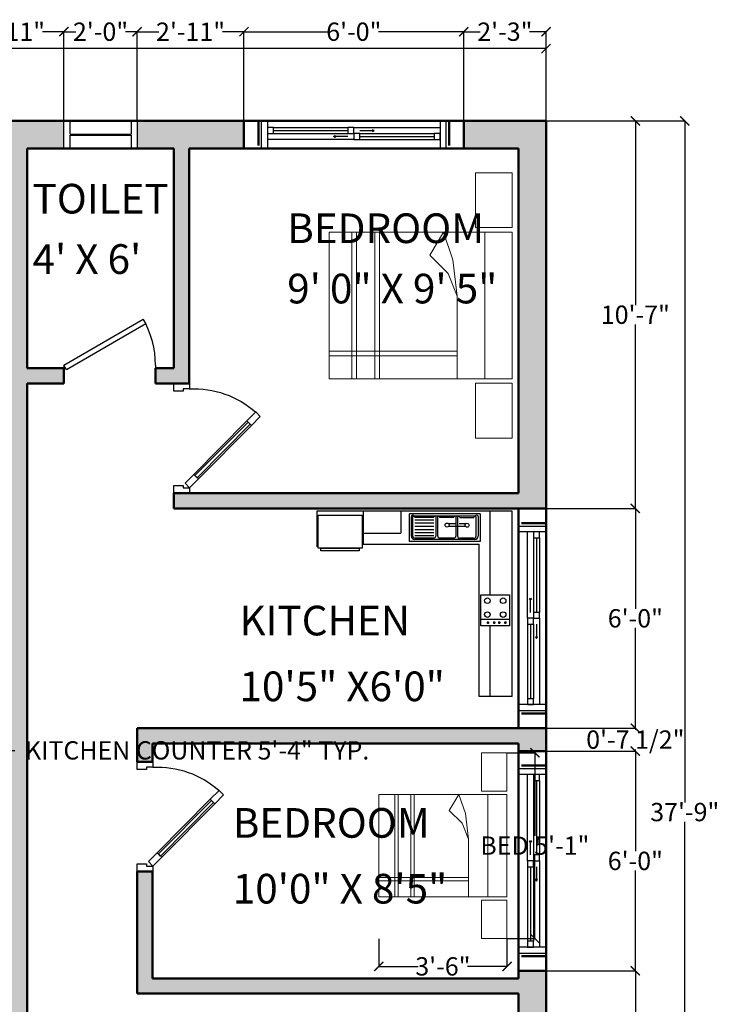
# Model space of a CAD drawing. Units: inches. Extents: x 2278 to 7495, y -71 to 1198.
# Tile 7 of 44: x 3076 to 3306, y 873 to 1195. Entities that reach past the tile are written whole.
import ezdxf

# ---------------------------------------------------------------- set-up
doc = ezdxf.new("R2010")
doc.units = ezdxf.units.IN
doc.header["$MEASUREMENT"] = 0
for name, color, linetype, lineweight in [('A-ANNO-DIMS', 2, 'Continuous', 18), ('A-AREA-IDEN', 3, 'Continuous', 18), ('A-Door', 3, 'Continuous', 25), ('A-FLOR-FIXT', 9, 'Continuous', 18), ('A-FURN', 8, 'Continuous', 18), ('A-Glaz', 4, 'Continuous', 25), ('A-Wall', 7, 'Continuous', 50), ('A-WALL-PATT', 8, 'Continuous', 18)]:
    doc.layers.add(name, color=color, linetype=linetype, lineweight=lineweight)
doc.layers.add('TEFRIŞ', color=11, linetype='Continuous')
doc.styles.get("Standard").update_dxf_attribs({"font": 'arial.ttf'})
doc.dimstyles.get("Standard").update_dxf_attribs({"dimtxt": 6, "dimasz": 3, "dimexe": 0.18, "dimexo": 0.0625, "dimgap": 0.09, "dimtad": 0, "dimtih": 1, "dimtoh": 1, "dimdec": 0, "dimzin": 0, "dimdsep": 46, "dimlunit": 3, "dimtxsty": 'Standard', "dimblk": 'ARCHTICK', "dimcen": 0.09, "dimadec": 0, "dimazin": 0, "dimtfac": 1, "dimtdec": 0, "dimtofl": 0, "dimtmove": 0, "dimatfit": 3, "dimfxl": 1, "dimtolj": 1, "dimtzin": 0, "dimarcsym": 0})

# ---------------------------------------------------------------- blocks, each defined once
blk = doc.blocks.new('A$C1DF4181C')
blk.add_lwpolyline([(120, 128), (460.7, 466.1), (432.5, 494.5), (91.8, 156.4)], close=True)
blk.add_arc((72.4, 128.7), 593.3, 357.23132, 41.49368)
at = {"layer": 'A-Door'}
for points in [[(517.5, 522.4), (460.7, 466.1), (432.5, 494.5), (489.3, 550.8)], [(63.2, 71.6), (120, 128), (91.8, 156.4), (35, 100)], [(35, 100), (0, 100), (0, 0), (50, 0), (50, 50), (50, 60), (35, 60)], [(665, 100), (665, 60), (650, 60), (650, 50), (650, 0), (700, 0), (700, 100)]]:
    blk.add_lwpolyline(points, close=True, dxfattribs=at)
at = {"layer": 'A-Glaz'}
blk.add_lwpolyline([(112.9, 135.1), (453.6, 473.2), (439.5, 487.4), (98.8, 149.3)], close=True, dxfattribs=at)
at = {"layer": 'A-Wall'}
for p, q in [((0, 0), (0, 100)), ((0, 100), (0, 0)), ((700, 0), (700, 100)), ((700, 0), (700, 100))]:
    blk.add_line(p, q, dxfattribs=at)
blk = doc.blocks.new('*U4')
for p, q in [((0, 0), (0, -6)), ((30, 0), (30, -6))]:
    blk.add_line(p, q)
blk.add_lwpolyline([(0, 0), (25.98, 15), (26.86, 13.48), (0.87, -1.52)], close=True)
blk.add_arc((0, 0), 30, 0, 30)
blk = doc.blocks.new('BED-160')
at = {"color": 0}
for p, q in [((-0.45, 2.35), (-0.45, 2.95)), ((-0.45, 2.95), (-0.05, 2.95)), ((-0.05, 2.95), (-0.05, 2.35)), ((-2.05, 2.3), (-0.05, 2.3)), ((-2.05, 0.7), (-2.05, 2.3)), ((-1.8, 0.7), (-1.8, 2.3)), ((-1.75, 0.7), (-1.75, 2.3)), ((-1.55, 0.7), (-1.55, 2.3)), ((-1.5, 0.7), (-1.5, 2.3)), ((-0.8, 2.3), (-0.95, 2.05)), ((-0.8, 2.3), (-0.7, 2)), ((-0.05, 2.35), (-0.45, 2.35)), ((-0.35, 0.7), (-0.35, 2.3)), ((-0.05, 2.3), (-0.05, 0.7)), ((-0.95, 2.05), (-0.75, 1.85)), ((-0.7, 2), (-0.65, 1.6)), ((-0.75, 1.85), (-0.65, 1.6)), ((-0.65, 1.6), (-0.65, 0.7)), ((-0.65, 1), (-2.05, 1)), ((-0.65, 0.95), (-2.05, 0.95)), ((-0.05, 0.7), (-2.05, 0.7)), ((-0.45, 0.65), (-0.05, 0.65)), ((-0.45, 0.05), (-0.45, 0.65)), ((-0.05, 0.65), (-0.05, 0.05)), ((-0.05, 0.05), (-0.45, 0.05))]:
    blk.add_line(p, q, dxfattribs=at)
blk = doc.blocks.new('A$C008029BD')
at = {"layer": 'TEFRIŞ', "ltscale": 0.05}
for p, q in [((0, 0), (0, -3.55)), ((3.37, 0), (0, 0)), ((3.37, 0), (3.37, -0.6)), ((1.522, -0.4), (0, -0.4)), ((3.37, -0.4), (2.083, -0.4)), ((0.05, -0.581), (0.05, -1.869)), ((0.05, -0.581), (0.55, -0.581)), ((0.086, -1.773), (0.086, -0.677)), ((0.096, -0.617), (0.454, -0.617)), ((0.099, -0.659), (0.457, -0.659)), ((0.113, -0.954), (0.113, -0.695)), ((0.493, -0.695), (0.493, -0.954)), ((0.514, -0.677), (0.514, -1.773)), ((0.55, -0.581), (0.55, -1.869)), ((0.6, -2.71), (0.6, -0.6)), ((3.37, -0.6), (0.6, -0.6)), ((0.23, -0.846), (0.229, -0.967)), ((0.28, -0.846), (0.277, -1.158)), ((0.096, -1.024), (0.454, -1.024)), ((0.457, -0.99), (0.099, -0.99)), ((0.11, -1.319), (0.11, -1.06)), ((0.228, -1.02), (0.227, -1.159)), ((0.49, -1.06), (0.49, -1.319)), ((0.454, -1.355), (0.096, -1.355)), ((0.096, -1.391), (0.454, -1.391)), ((0.11, -1.773), (0.11, -1.427)), ((0.154, -1.773), (0.154, -1.427)), ((0.214, -1.773), (0.214, -1.427)), ((0.274, -1.773), (0.274, -1.427)), ((0.334, -1.773), (0.334, -1.427)), ((0.39, -1.773), (0.39, -1.427)), ((0.444, -1.773), (0.444, -1.427)), ((0.49, -1.427), (0.49, -1.773)), ((0.55, -1.869), (0.05, -1.869)), ((0.454, -1.809), (0.096, -1.809)), ((0.454, -1.833), (0.096, -1.833)), ((0, -2.025), (0.4, -2.025)), ((0.4, -2.71), (0.4, -2.025)), ((0, -2.71), (0.6, -2.71)), ((0, -3.55), (0.65, -3.55))]:
    blk.add_line(p, q, dxfattribs=at)
at = {"layer": 'TEFRIŞ'}
blk.add_line((1.969, -0.05), (1.969, -0.572), dxfattribs=at)
at = {"layer": 'TEFRIŞ', "ltscale": 0.05}
for points in [[(1.522, -0.05), (2.083, -0.05), (2.083, -0.572), (1.522, -0.572)], [(0.67, -2.73), (0.67, -3.53), (0.07, -3.53), (0.07, -2.73)], [(0.72, -2.78), (0.72, -3.48), (0.67, -3.48), (0.67, -2.78)]]:
    blk.add_lwpolyline(points, close=True, dxfattribs=at)
at = {"layer": 'TEFRIŞ', "const_width": 0.025}
for points in [[(2.014, -0.123, 1), (2.039, -0.123, 1)], [(2.014, -0.236, 1), (2.039, -0.236, 1)], [(2.014, -0.327, 1), (2.039, -0.327, 1)], [(2.014, -0.44, 1), (2.039, -0.44, 1)]]:
    blk.add_lwpolyline(points, format="xyb", close=True, dxfattribs=at)
at = {"layer": 'TEFRIŞ', "ltscale": 0.05}
for centre, radius in [((1.628, -0.164), 0.0505), ((1.628, -0.45), 0.0505), ((0.255, -0.82), 0.036), ((0.252, -1.184), 0.036)]:
    blk.add_circle(centre, radius, dxfattribs=at)
at = {"layer": 'TEFRIŞ'}
for centre in [(1.88, -0.164), (1.88, -0.45)]:
    blk.add_circle(centre, 0.0505, dxfattribs=at)
at = {"layer": 'TEFRIŞ', "ltscale": 0.05}
for centre, radius, start, end in [((0.108, -0.649), 0.0351, 110.4976, 230.5777), ((0.118, -0.673), 0.023, 143.9853, 258.5157), ((0.454, -0.677), 0.06, 0, 90), ((0.457, -0.695), 0.036, 0, 90), ((0.115, -1.038), 0.023, 143.9853, 258.5157), ((0.118, -0.976), 0.023, 101.4843, 216.0147), ((0.454, -1.06), 0.036, 0, 90), ((0.457, -0.954), 0.036, 270, 0), ((0.115, -1.341), 0.023, 101.4843, 216.0147), ((0.115, -1.405), 0.023, 143.9853, 258.5157), ((0.454, -1.319), 0.036, 270, 0), ((0.454, -1.427), 0.036, 0, 90), ((0.108, -1.801), 0.0351, 129.4223, 249.5024), ((0.115, -1.796), 0.023, 101.4843, 216.0147), ((0.454, -1.773), 0.06, 270, 0), ((0.454, -1.773), 0.036, 270, 0)]:
    blk.add_arc(centre, radius, start, end, dxfattribs=at)
blk = doc.blocks.new('_ArchTick')
at = {"color": 0, "linetype": 'ByBlock', "const_width": 0.15}
blk.add_lwpolyline([(-0.5, -0.5), (0.5, 0.5)], dxfattribs=at)
blk = doc.blocks.new('*D35')
at = {"layer": 'A-ANNO-DIMS', "color": 0, "lineweight": -2, "transparency": 16777216}
for p, q in [((3248.99, 1162.26), (3294.56, 1162.26)), ((3294.38, 1162.26), (3294.38, 938.91)), ((3294.38, 709.26), (3294.38, 932.6)), ((3248.99, 709.26), (3294.56, 709.26))]:
    blk.add_line(p, q, dxfattribs=at)
at = {"layer": 'Defpoints', "color": 0, "transparency": 16777216}
for p in [(3248.93, 1162.26), (3248.93, 709.26), (3294.38, 709.26)]:
    blk.add_point(p, dxfattribs=at)
at = {"layer": 'A-ANNO-DIMS', "color": 0, "lineweight": -2, "transparency": 16777216, "xscale": 3, "yscale": 3, "zscale": 3}
for p, rotation in [((3294.38, 1162.26), 90), ((3294.38, 709.26), 270)]:
    blk.add_blockref('_ArchTick', p, dxfattribs=dict(at, rotation=rotation))
at = {"layer": 'A-ANNO-DIMS', "color": 0, "transparency": 16777216, "insert": (3294.38, 935.76), "char_height": 6, "attachment_point": 5}
blk.add_mtext('\\A1;37\'-9"', dxfattribs=at)
blk = doc.blocks.new('*D36')
at = {"layer": 'A-ANNO-DIMS', "color": 0, "lineweight": -2, "transparency": 16777216}
for p, q in [((2845.93, 1162.32), (2845.93, 1186.15)), ((2845.93, 1185.97), (3037.04, 1185.97)), ((3248.93, 1185.97), (3057.82, 1185.97)), ((3248.93, 1162.32), (3248.93, 1186.15))]:
    blk.add_line(p, q, dxfattribs=at)
at = {"layer": 'Defpoints', "color": 0, "transparency": 16777216}
for p in [(3248.93, 1185.97), (2845.93, 1162.26), (3248.93, 1162.26)]:
    blk.add_point(p, dxfattribs=at)
at = {"layer": 'A-ANNO-DIMS', "color": 0, "lineweight": -2, "transparency": 16777216, "xscale": 3, "yscale": 3, "zscale": 3, "rotation": 180}
blk.add_blockref('_ArchTick', (2845.93, 1185.97), dxfattribs=at)
at = {"layer": 'A-ANNO-DIMS', "color": 0, "lineweight": -2, "transparency": 16777216, "xscale": 3, "yscale": 3, "zscale": 3}
blk.add_blockref('_ArchTick', (3248.93, 1185.97), dxfattribs=at)
at = {"layer": 'A-ANNO-DIMS', "color": 0, "transparency": 16777216, "insert": (3047.43, 1185.97), "char_height": 6, "attachment_point": 5}
blk.add_mtext('\\A1;33\'-7"', dxfattribs=at)
blk = doc.blocks.new('*D51')
at = {"layer": 'A-ANNO-DIMS', "color": 0, "lineweight": -2, "transparency": 16777216}
for p, q in [((3236.18, 955.22), (3245.43, 955.22)), ((3245.25, 955.22), (3245.25, 927.93)), ((3245.25, 894.32), (3245.25, 921.62)), ((3236.18, 894.32), (3245.43, 894.32))]:
    blk.add_line(p, q, dxfattribs=at)
at = {"layer": 'Defpoints', "color": 0, "transparency": 16777216}
for p in [(3236.12, 955.22), (3245.25, 955.22), (3236.12, 894.32)]:
    blk.add_point(p, dxfattribs=at)
at = {"layer": 'A-ANNO-DIMS', "color": 0, "lineweight": -2, "transparency": 16777216, "xscale": 3, "yscale": 3, "zscale": 3}
for p, rotation in [((3245.25, 955.22), 90), ((3245.25, 894.32), 270)]:
    blk.add_blockref('_ArchTick', p, dxfattribs=dict(at, rotation=rotation))
at = {"layer": 'A-ANNO-DIMS', "color": 0, "transparency": 16777216, "insert": (3245.25, 924.77), "char_height": 6, "attachment_point": 5}
blk.add_mtext('\\A1;BED 5\'-1"', dxfattribs=at)
blk = doc.blocks.new('*D52')
at = {"layer": 'A-ANNO-DIMS', "color": 0, "lineweight": -2, "transparency": 16777216}
for p, q in [((3194.12, 894.26), (3194.12, 885.01)), ((3236.12, 894.26), (3236.12, 885.01)), ((3194.12, 885.19), (3207.06, 885.19)), ((3236.12, 885.19), (3223.18, 885.19))]:
    blk.add_line(p, q, dxfattribs=at)
at = {"layer": 'Defpoints', "color": 0, "transparency": 16777216}
for p in [(3194.12, 894.32), (3236.12, 894.32), (3236.12, 885.19)]:
    blk.add_point(p, dxfattribs=at)
at = {"layer": 'A-ANNO-DIMS', "color": 0, "lineweight": -2, "transparency": 16777216, "xscale": 3, "yscale": 3, "zscale": 3, "rotation": 180}
blk.add_blockref('_ArchTick', (3194.12, 885.19), dxfattribs=at)
at = {"layer": 'A-ANNO-DIMS', "color": 0, "lineweight": -2, "transparency": 16777216, "xscale": 3, "yscale": 3, "zscale": 3}
blk.add_blockref('_ArchTick', (3236.12, 885.19), dxfattribs=at)
at = {"layer": 'A-ANNO-DIMS', "color": 0, "transparency": 16777216, "insert": (3215.12, 885.19), "char_height": 6, "attachment_point": 5}
blk.add_mtext('\\A1;3\'-6"', dxfattribs=at)
blk = doc.blocks.new('*D53')
at = {"layer": 'A-ANNO-DIMS', "color": 0, "lineweight": -2, "transparency": 16777216}
for p, q in [((3007.93, 965.51), (3007.93, 955.8)), ((3071.89, 965.51), (3071.89, 955.8)), ((3007.93, 955.98), (3071.89, 955.98)), ((3071.89, 955.98), (3074.89, 955.98))]:
    blk.add_line(p, q, dxfattribs=at)
at = {"layer": 'Defpoints', "color": 0, "transparency": 16777216}
for p in [(3007.93, 965.57), (3071.89, 965.57), (3071.89, 955.98)]:
    blk.add_point(p, dxfattribs=at)
at = {"layer": 'A-ANNO-DIMS', "color": 0, "lineweight": -2, "transparency": 16777216, "xscale": 3, "yscale": 3, "zscale": 3, "rotation": 180}
blk.add_blockref('_ArchTick', (3007.93, 955.98), dxfattribs=at)
at = {"layer": 'A-ANNO-DIMS', "color": 0, "lineweight": -2, "transparency": 16777216, "xscale": 3, "yscale": 3, "zscale": 3}
blk.add_blockref('_ArchTick', (3071.89, 955.98), dxfattribs=at)
at = {"layer": 'A-ANNO-DIMS', "color": 0, "transparency": 16777216, "insert": (3134.58, 955.98), "char_height": 6, "attachment_point": 5}
blk.add_mtext('\\A1;KITCHEN COUNTER 5\'-4" TYP.', dxfattribs=at)
blk = doc.blocks.new('*D81')
at = {"layer": 'A-ANNO-DIMS', "color": 0, "lineweight": -2, "transparency": 16777216}
for p, q in [((3055.93, 1162.32), (3055.93, 1191.69)), ((3055.93, 1191.51), (3062.98, 1191.51)), ((3090.93, 1191.51), (3083.88, 1191.51)), ((3090.93, 1162.32), (3090.93, 1191.69))]:
    blk.add_line(p, q, dxfattribs=at)
at = {"layer": 'Defpoints', "color": 0, "transparency": 16777216}
for p in [(3090.93, 1191.51), (3055.93, 1162.26), (3090.93, 1162.26)]:
    blk.add_point(p, dxfattribs=at)
at = {"layer": 'A-ANNO-DIMS', "color": 0, "lineweight": -2, "transparency": 16777216, "xscale": 3, "yscale": 3, "zscale": 3, "rotation": 180}
blk.add_blockref('_ArchTick', (3055.93, 1191.51), dxfattribs=at)
at = {"layer": 'A-ANNO-DIMS', "color": 0, "lineweight": -2, "transparency": 16777216, "xscale": 3, "yscale": 3, "zscale": 3}
blk.add_blockref('_ArchTick', (3090.93, 1191.51), dxfattribs=at)
at = {"layer": 'A-ANNO-DIMS', "color": 0, "transparency": 16777216, "insert": (3073.43, 1191.51), "char_height": 6, "attachment_point": 5}
blk.add_mtext('\\A1;2\'-11"', dxfattribs=at)
blk = doc.blocks.new('*D82')
at = {"layer": 'A-ANNO-DIMS', "color": 0, "lineweight": -2, "transparency": 16777216}
for p, q in [((3090.93, 1162.32), (3090.93, 1191.69)), ((3090.93, 1191.51), (3094.81, 1191.51)), ((3114.93, 1191.51), (3111.05, 1191.51)), ((3114.93, 1162.32), (3114.93, 1191.69))]:
    blk.add_line(p, q, dxfattribs=at)
at = {"layer": 'Defpoints', "color": 0, "transparency": 16777216}
for p in [(3114.93, 1191.51), (3090.93, 1162.26), (3114.93, 1162.26)]:
    blk.add_point(p, dxfattribs=at)
at = {"layer": 'A-ANNO-DIMS', "color": 0, "lineweight": -2, "transparency": 16777216, "xscale": 3, "yscale": 3, "zscale": 3, "rotation": 180}
blk.add_blockref('_ArchTick', (3090.93, 1191.51), dxfattribs=at)
at = {"layer": 'A-ANNO-DIMS', "color": 0, "lineweight": -2, "transparency": 16777216, "xscale": 3, "yscale": 3, "zscale": 3}
blk.add_blockref('_ArchTick', (3114.93, 1191.51), dxfattribs=at)
at = {"layer": 'A-ANNO-DIMS', "color": 0, "transparency": 16777216, "insert": (3102.93, 1191.51), "char_height": 6, "attachment_point": 5}
blk.add_mtext('\\A1;2\'-0"', dxfattribs=at)
blk = doc.blocks.new('*D83')
at = {"layer": 'A-ANNO-DIMS', "color": 0, "lineweight": -2, "transparency": 16777216}
for p, q in [((3114.93, 1162.32), (3114.93, 1191.69)), ((3114.93, 1191.51), (3121.98, 1191.51)), ((3149.93, 1191.51), (3142.88, 1191.51)), ((3149.93, 1162.32), (3149.93, 1191.69))]:
    blk.add_line(p, q, dxfattribs=at)
at = {"layer": 'Defpoints', "color": 0, "transparency": 16777216}
for p in [(3149.93, 1191.51), (3114.93, 1162.26), (3149.93, 1162.26)]:
    blk.add_point(p, dxfattribs=at)
at = {"layer": 'A-ANNO-DIMS', "color": 0, "lineweight": -2, "transparency": 16777216, "xscale": 3, "yscale": 3, "zscale": 3, "rotation": 180}
blk.add_blockref('_ArchTick', (3114.93, 1191.51), dxfattribs=at)
at = {"layer": 'A-ANNO-DIMS', "color": 0, "lineweight": -2, "transparency": 16777216, "xscale": 3, "yscale": 3, "zscale": 3}
blk.add_blockref('_ArchTick', (3149.93, 1191.51), dxfattribs=at)
at = {"layer": 'A-ANNO-DIMS', "color": 0, "transparency": 16777216, "insert": (3132.43, 1191.51), "char_height": 6, "attachment_point": 5}
blk.add_mtext('\\A1;2\'-11"', dxfattribs=at)
blk = doc.blocks.new('*D84')
at = {"layer": 'A-ANNO-DIMS', "color": 0, "lineweight": -2, "transparency": 16777216}
for p, q in [((3149.93, 1162.32), (3149.93, 1191.69)), ((3149.93, 1191.51), (3177.85, 1191.51)), ((3221.93, 1191.51), (3194.01, 1191.51)), ((3221.93, 1162.32), (3221.93, 1191.69))]:
    blk.add_line(p, q, dxfattribs=at)
at = {"layer": 'Defpoints', "color": 0, "transparency": 16777216}
for p in [(3221.93, 1191.51), (3149.93, 1162.26), (3221.93, 1162.26)]:
    blk.add_point(p, dxfattribs=at)
at = {"layer": 'A-ANNO-DIMS', "color": 0, "lineweight": -2, "transparency": 16777216, "xscale": 3, "yscale": 3, "zscale": 3, "rotation": 180}
blk.add_blockref('_ArchTick', (3149.93, 1191.51), dxfattribs=at)
at = {"layer": 'A-ANNO-DIMS', "color": 0, "lineweight": -2, "transparency": 16777216, "xscale": 3, "yscale": 3, "zscale": 3}
blk.add_blockref('_ArchTick', (3221.93, 1191.51), dxfattribs=at)
at = {"layer": 'A-ANNO-DIMS', "color": 0, "transparency": 16777216, "insert": (3185.93, 1191.51), "char_height": 6, "attachment_point": 5}
blk.add_mtext('\\A1;6\'-0"', dxfattribs=at)
blk = doc.blocks.new('*D85')
at = {"layer": 'A-ANNO-DIMS', "color": 0, "lineweight": -2, "transparency": 16777216}
for p, q in [((3221.93, 1162.32), (3221.93, 1191.69)), ((3221.93, 1191.51), (3227.31, 1191.51)), ((3248.93, 1191.51), (3243.55, 1191.51)), ((3248.93, 1162.32), (3248.93, 1191.69))]:
    blk.add_line(p, q, dxfattribs=at)
at = {"layer": 'Defpoints', "color": 0, "transparency": 16777216}
for p in [(3248.93, 1191.51), (3221.93, 1162.26), (3248.93, 1162.26)]:
    blk.add_point(p, dxfattribs=at)
at = {"layer": 'A-ANNO-DIMS', "color": 0, "lineweight": -2, "transparency": 16777216, "xscale": 3, "yscale": 3, "zscale": 3, "rotation": 180}
blk.add_blockref('_ArchTick', (3221.93, 1191.51), dxfattribs=at)
at = {"layer": 'A-ANNO-DIMS', "color": 0, "lineweight": -2, "transparency": 16777216, "xscale": 3, "yscale": 3, "zscale": 3}
blk.add_blockref('_ArchTick', (3248.93, 1191.51), dxfattribs=at)
at = {"layer": 'A-ANNO-DIMS', "color": 0, "transparency": 16777216, "insert": (3235.43, 1191.51), "char_height": 6, "attachment_point": 5}
blk.add_mtext('\\A1;2\'-3"', dxfattribs=at)
blk = doc.blocks.new('*D86')
at = {"layer": 'A-ANNO-DIMS', "color": 0, "lineweight": -2, "transparency": 16777216}
for p, q in [((3248.99, 1162.26), (3278.36, 1162.26)), ((3278.18, 1162.26), (3278.18, 1101.91)), ((3278.18, 1035.26), (3278.18, 1095.6)), ((3248.99, 1035.26), (3278.36, 1035.26))]:
    blk.add_line(p, q, dxfattribs=at)
at = {"layer": 'Defpoints', "color": 0, "transparency": 16777216}
for p in [(3248.93, 1162.26), (3248.93, 1035.26), (3278.18, 1035.26)]:
    blk.add_point(p, dxfattribs=at)
at = {"layer": 'A-ANNO-DIMS', "color": 0, "lineweight": -2, "transparency": 16777216, "xscale": 3, "yscale": 3, "zscale": 3}
for p, rotation in [((3278.18, 1162.26), 90), ((3278.18, 1035.26), 270)]:
    blk.add_blockref('_ArchTick', p, dxfattribs=dict(at, rotation=rotation))
at = {"layer": 'A-ANNO-DIMS', "color": 0, "transparency": 16777216, "insert": (3278.18, 1098.76), "char_height": 6, "attachment_point": 5}
blk.add_mtext('\\A1;10\'-7"', dxfattribs=at)
blk = doc.blocks.new('*D87')
at = {"layer": 'A-ANNO-DIMS', "color": 0, "lineweight": -2, "transparency": 16777216}
for p, q in [((3248.99, 1035.26), (3278.36, 1035.26)), ((3278.18, 1035.26), (3278.18, 1002.41)), ((3278.18, 963.26), (3278.18, 996.1)), ((3248.99, 963.26), (3278.36, 963.26))]:
    blk.add_line(p, q, dxfattribs=at)
at = {"layer": 'Defpoints', "color": 0, "transparency": 16777216}
for p in [(3248.93, 1035.26), (3248.93, 963.26), (3278.18, 963.26)]:
    blk.add_point(p, dxfattribs=at)
at = {"layer": 'A-ANNO-DIMS', "color": 0, "lineweight": -2, "transparency": 16777216, "xscale": 3, "yscale": 3, "zscale": 3}
for p, rotation in [((3278.18, 1035.26), 90), ((3278.18, 963.26), 270)]:
    blk.add_blockref('_ArchTick', p, dxfattribs=dict(at, rotation=rotation))
at = {"layer": 'A-ANNO-DIMS', "color": 0, "transparency": 16777216, "insert": (3278.18, 999.26), "char_height": 6, "attachment_point": 5}
blk.add_mtext('\\A1;6\'-0"', dxfattribs=at)
blk = doc.blocks.new('*D88')
at = {"layer": 'A-ANNO-DIMS', "color": 0, "lineweight": -2, "transparency": 16777216}
for p, q in [((3248.99, 963.26), (3278.36, 963.26)), ((3278.18, 963.26), (3278.18, 962.7)), ((3248.99, 955.76), (3278.36, 955.76)), ((3278.18, 955.76), (3278.18, 956.31))]:
    blk.add_line(p, q, dxfattribs=at)
at = {"layer": 'Defpoints', "color": 0, "transparency": 16777216}
for p in [(3248.93, 963.26), (3248.93, 955.76), (3278.18, 955.76)]:
    blk.add_point(p, dxfattribs=at)
at = {"layer": 'A-ANNO-DIMS', "color": 0, "lineweight": -2, "transparency": 16777216, "xscale": 3, "yscale": 3, "zscale": 3}
for p, rotation in [((3278.18, 963.26), 90), ((3278.18, 955.76), 270)]:
    blk.add_blockref('_ArchTick', p, dxfattribs=dict(at, rotation=rotation))
at = {"layer": 'A-ANNO-DIMS', "color": 0, "transparency": 16777216, "insert": (3278.18, 959.51), "char_height": 6, "attachment_point": 5}
blk.add_mtext('\\A1;0\'-7 1/2"', dxfattribs=at)
blk = doc.blocks.new('*D89')
at = {"layer": 'A-ANNO-DIMS', "color": 0, "lineweight": -2, "transparency": 16777216}
for p, q in [((3248.99, 955.76), (3278.36, 955.76)), ((3278.18, 955.76), (3278.18, 922.91)), ((3278.18, 883.76), (3278.18, 916.6)), ((3248.99, 883.76), (3278.36, 883.76))]:
    blk.add_line(p, q, dxfattribs=at)
at = {"layer": 'Defpoints', "color": 0, "transparency": 16777216}
for p in [(3248.93, 955.76), (3248.93, 883.76), (3278.18, 883.76)]:
    blk.add_point(p, dxfattribs=at)
at = {"layer": 'A-ANNO-DIMS', "color": 0, "lineweight": -2, "transparency": 16777216, "xscale": 3, "yscale": 3, "zscale": 3}
for p, rotation in [((3278.18, 955.76), 90), ((3278.18, 883.76), 270)]:
    blk.add_blockref('_ArchTick', p, dxfattribs=dict(at, rotation=rotation))
at = {"layer": 'A-ANNO-DIMS', "color": 0, "transparency": 16777216, "insert": (3278.18, 919.76), "char_height": 6, "attachment_point": 5}
blk.add_mtext('\\A1;6\'-0"', dxfattribs=at)
blk = doc.blocks.new('*D90')
at = {"layer": 'A-ANNO-DIMS', "color": 0, "lineweight": -2, "transparency": 16777216}
for p, q in [((3248.99, 883.76), (3278.36, 883.76)), ((3278.18, 883.76), (3278.18, 799.7)), ((3278.18, 709.26), (3278.18, 793.31)), ((3248.99, 709.26), (3278.36, 709.26))]:
    blk.add_line(p, q, dxfattribs=at)
at = {"layer": 'Defpoints', "color": 0, "transparency": 16777216}
for p in [(3248.93, 883.76), (3248.93, 709.26), (3278.18, 709.26)]:
    blk.add_point(p, dxfattribs=at)
at = {"layer": 'A-ANNO-DIMS', "color": 0, "lineweight": -2, "transparency": 16777216, "xscale": 3, "yscale": 3, "zscale": 3}
for p, rotation in [((3278.18, 883.76), 90), ((3278.18, 709.26), 270)]:
    blk.add_blockref('_ArchTick', p, dxfattribs=dict(at, rotation=rotation))
at = {"layer": 'A-ANNO-DIMS', "color": 0, "transparency": 16777216, "insert": (3278.18, 796.51), "char_height": 6, "attachment_point": 5}
blk.add_mtext('\\A1;14\'-6 1/2"', dxfattribs=at)

msp = doc.modelspace()

# ---------------------------------------------------------------- hatches: boundary and pattern name
at = {"layer": 'A-WALL-PATT', "transparency": 33554687}
h = msp.add_hatch(dxfattribs=at)
h.set_pattern_fill('ANSI36', color=256, scale=30)
h.paths.add_polyline_path([(3248.93, 883.76), (3239.93, 883.76), (3239.93, 881.26), (3119.93, 881.26), (3119.93, 916.26), (3114.93, 916.26), (3114.93, 876.26), (3239.93, 876.26), (3239.93, 759.26), (3195.43, 759.26), (3195.43, 754.26), (3248.93, 754.26)])
h.paths.add_polyline_path([(3248.93, 963.26), (3239.93, 963.26), (3114.93, 963.26), (3114.93, 952.26), (3119.93, 952.26), (3119.93, 958.26), (3239.93, 958.26), (3239.93, 955.76), (3248.93, 955.76)])
h.paths.add_polyline_path([(3078.93, 1076.26), (3090.93, 1076.26), (3090.93, 1081.26), (3078.93, 1081.26), (3078.93, 1153.26), (3090.93, 1153.26), (3090.93, 1162.26), (3055.93, 1162.26), (3055.93, 1153.26), (3073.93, 1153.26), (3073.93, 1033.26), (3007.93, 1033.26), (3007.93, 1028.26), (3073.93, 1028.26), (3073.93, 942.26), (3073.93, 938.92), (3073.93, 875.26), (3025.93, 875.26), (3025.93, 942.26), (3020.93, 942.26), (3020.93, 870.26), (3020.93, 864.53), (3025.94, 864.53), (3025.94, 870.26), (3073.93, 870.26), (3073.93, 804.26), (3078.93, 804.26)])
h.paths.add_polyline_path([(2983.93, 1162.26), (2943.93, 1162.26), (2943.93, 1153.26), (2960.93, 1153.26), (2960.93, 1033.26), (2960.93, 1028.26), (2965.93, 1028.26), (2965.93, 1153.26), (2983.93, 1153.26)])
h.paths.add_polyline_path([(3149.93, 1162.26), (3114.93, 1162.26), (3114.93, 1153.26), (3126.93, 1153.26), (3126.93, 1081.26), (3120.93, 1081.26), (3120.93, 1076.26), (3131.93, 1076.26), (3131.93, 1153.26), (3149.93, 1153.26)])
h.paths.add_polyline_path([(3248.93, 1162.26), (3221.93, 1162.26), (3221.93, 1153.26), (3239.93, 1153.26), (3239.93, 1040.26), (3126.93, 1040.26), (3126.93, 1035.26), (3239.93, 1035.26), (3248.93, 1035.26)])
h.paths.add_polyline_path([(3123.43, 759.26), (3078.93, 759.26), (3078.93, 762.26), (3073.93, 762.26), (3073.93, 754.26), (3123.43, 754.26)])
h.paths.add_polyline_path([(3025.93, 811.26), (3025.89, 817.61), (3020.93, 817.61), (3020.93, 811.26), (3008.93, 811.26), (3008.93, 806.26), (3025.93, 806.26)], flags=17)
h.paths.add_polyline_path([(2924.93, 1028.26), (2924.93, 1033.26), (2913.93, 1033.26), (2913.93, 1028.26), (2919.93, 1028.26), (2919.93, 956.26), (2899.18, 956.26), (2899.18, 951.26), (2924.93, 951.26)])
h.paths.add_polyline_path([(2924.93, 915.26), (2901.93, 915.26), (2901.93, 910.26), (2924.93, 910.26)])
h.paths.add_polyline_path([(3078.14, 1129.24), (3130.7, 1129.24), (3130.7, 1144.33), (3078.14, 1144.33)], flags=9)

# ---------------------------------------------------------------- linework, layer by layer
at = {"layer": 'A-Glaz'}
for p, q in [((3090.93, 1162.26), (3114.93, 1162.26)), ((3090.93, 1153.26), (3090.93, 1162.26)), ((3092.93, 1157.96), (3092.93, 1162.26)), ((3112.93, 1162.26), (3112.93, 1157.96)), ((3114.93, 1162.26), (3114.93, 1153.26)), ((3157.63, 1162.26), (3214.23, 1162.26)), ((3159.58, 1160.09), (3183.98, 1160.09)), ((3159.58, 1159.11), (3183.98, 1159.11)), ((3185.93, 1160.09), (3214.23, 1160.09)), ((3187.88, 1159.11), (3192.07, 1159.11)), ((3092.93, 1157.96), (3112.93, 1157.96)), ((3092.93, 1153.26), (3092.93, 1157.56)), ((3092.93, 1157.56), (3112.93, 1157.56)), ((3112.93, 1157.56), (3112.93, 1153.26)), ((3185.93, 1156.18), (3157.63, 1156.18)), ((3159.58, 1158.14), (3183.98, 1158.14)), ((3183.98, 1157.16), (3179.79, 1157.16)), ((3187.88, 1158.14), (3212.28, 1158.14)), ((3187.88, 1157.16), (3212.28, 1157.16)), ((3187.88, 1156.18), (3212.28, 1156.18)), ((3114.93, 1153.26), (3090.93, 1153.26)), ((3157.63, 1153.26), (3214.23, 1153.26)), ((3239.93, 1027.56), (3239.93, 970.96)), ((3242.86, 999.26), (3242.86, 1027.56)), ((3248.93, 1027.56), (3248.93, 970.96)), ((3244.81, 1025.61), (3244.81, 1001.21)), ((3245.79, 1025.61), (3245.79, 1001.21)), ((3246.76, 1025.61), (3246.76, 1001.21)), ((3243.83, 1001.21), (3243.83, 1005.4)), ((3242.86, 997.31), (3242.86, 972.91)), ((3243.83, 997.31), (3243.83, 972.91)), ((3244.81, 997.31), (3244.81, 972.91)), ((3245.79, 997.31), (3245.79, 993.11)), ((3246.76, 999.26), (3246.76, 970.96)), ((3239.93, 948.06), (3239.93, 891.46)), ((3242.86, 919.76), (3242.86, 948.06)), ((3244.81, 946.11), (3244.81, 921.71)), ((3245.79, 946.11), (3245.79, 921.71)), ((3246.76, 946.11), (3246.76, 921.71)), ((3248.93, 948.06), (3248.93, 891.46)), ((3243.83, 921.71), (3243.83, 925.9)), ((3246.76, 919.76), (3246.76, 891.46)), ((3242.86, 917.81), (3242.86, 893.41)), ((3243.83, 917.81), (3243.83, 893.41)), ((3244.81, 917.81), (3244.81, 893.41)), ((3245.79, 917.81), (3245.79, 913.61))]:
    msp.add_line(p, q, dxfattribs=at)
for points in [[(3157.63, 1153.26), (3155.68, 1153.26), (3155.68, 1162.26), (3157.63, 1162.26)], [(3214.23, 1153.26), (3216.18, 1153.26), (3216.18, 1162.26), (3214.23, 1162.26)], [(3157.63, 1158.14), (3159.58, 1158.14), (3159.58, 1160.09), (3157.63, 1160.09)], [(3183.98, 1158.14), (3185.93, 1158.14), (3185.93, 1160.09), (3183.98, 1160.09)], [(3192.58, 1159.11), (3192.07, 1159.4), (3192.07, 1158.82)], [(3179.28, 1157.16), (3179.79, 1157.45), (3179.79, 1156.87)], [(3185.93, 1156.18), (3187.88, 1156.18), (3187.88, 1158.14), (3185.93, 1158.14)], [(3212.28, 1156.18), (3214.23, 1156.18), (3214.23, 1158.14), (3212.28, 1158.14)], [(3239.93, 1027.56), (3239.93, 1029.51), (3248.93, 1029.51), (3248.93, 1027.56)], [(3244.81, 1027.56), (3244.81, 1025.61), (3246.76, 1025.61), (3246.76, 1027.56)], [(3243.83, 1005.91), (3244.13, 1005.4), (3243.54, 1005.4)], [(3244.81, 1001.21), (3244.81, 999.26), (3246.76, 999.26), (3246.76, 1001.21)], [(3242.86, 999.26), (3242.86, 997.31), (3244.81, 997.31), (3244.81, 999.26)], [(3245.79, 992.61), (3246.08, 993.11), (3245.49, 993.11)], [(3242.86, 972.91), (3242.86, 970.96), (3244.81, 970.96), (3244.81, 972.91)], [(3239.93, 970.96), (3239.93, 969.01), (3248.93, 969.01), (3248.93, 970.96)], [(3239.93, 948.06), (3239.93, 950.01), (3248.93, 950.01), (3248.93, 948.06)], [(3244.81, 948.06), (3244.81, 946.11), (3246.76, 946.11), (3246.76, 948.06)], [(3243.83, 926.41), (3244.13, 925.9), (3243.54, 925.9)], [(3242.86, 919.76), (3242.86, 917.81), (3244.81, 917.81), (3244.81, 919.76)], [(3244.81, 921.71), (3244.81, 919.76), (3246.76, 919.76), (3246.76, 921.71)], [(3245.79, 913.11), (3246.08, 913.61), (3245.49, 913.61)], [(3239.93, 891.46), (3239.93, 889.51), (3248.93, 889.51), (3248.93, 891.46)], [(3242.86, 893.41), (3242.86, 891.46), (3244.81, 891.46), (3244.81, 893.41)]]:
    msp.add_lwpolyline(points, close=True, dxfattribs=at)
at = {"layer": 'A-Wall'}
for p, q in [((2845.93, 1162.26), (3248.93, 1162.26)), ((3149.93, 1153.26), (3149.93, 1162.26)), ((3155.68, 1162.26), (3149.93, 1162.26)), ((3154.7, 1162.04), (3154.7, 1154.23)), ((3216.18, 1162.26), (3221.93, 1162.26)), ((3217.16, 1162.04), (3217.16, 1154.23)), ((3221.93, 1153.26), (3221.93, 1162.26)), ((3248.93, 1162.26), (3248.93, 713.26)), ((3078.93, 1153.26), (3078.93, 1081.26)), ((3078.93, 1153.26), (3126.93, 1153.26)), ((3126.93, 1153.26), (3126.93, 1081.26)), ((3131.93, 1153.26), (3131.93, 1076.26)), ((3131.93, 1153.26), (3239.93, 1153.26)), ((3155.68, 1153.26), (3149.93, 1153.26)), ((3216.18, 1153.26), (3221.93, 1153.26)), ((3239.93, 1153.26), (3239.93, 1040.26)), ((3078.93, 1081.26), (3090.93, 1081.26)), ((3090.93, 1076.26), (3090.93, 1081.26)), ((3120.93, 1081.26), (3126.93, 1081.26)), ((3120.93, 1076.26), (3120.93, 1081.26)), ((3078.93, 1076.26), (3078.93, 804.26)), ((3078.93, 1076.26), (3090.93, 1076.26)), ((3120.93, 1076.26), (3131.93, 1076.26)), ((3126.93, 1040.26), (3126.93, 1035.26)), ((3126.93, 1040.26), (3239.93, 1040.26)), ((3126.93, 1035.26), (3239.93, 1035.26)), ((3239.93, 1035.26), (3239.93, 963.26)), ((3239.93, 1035.26), (3248.93, 1035.26)), ((3239.93, 1029.51), (3239.93, 1035.26)), ((3248.93, 1029.51), (3248.93, 1035.26)), ((3248.71, 1030.48), (3240.91, 1030.48)), ((3239.93, 969.01), (3239.93, 963.26)), ((3248.93, 969.01), (3248.93, 963.26)), ((3248.71, 968.03), (3240.91, 968.03)), ((3114.93, 963.26), (3239.93, 963.26)), ((3114.93, 963.26), (3114.93, 952.26)), ((3239.93, 963.26), (3248.93, 963.26)), ((3119.93, 958.26), (3239.93, 958.26)), ((3119.93, 958.26), (3119.93, 952.26)), ((3239.93, 958.26), (3239.93, 881.26)), ((3239.93, 955.76), (3248.93, 955.76)), ((3239.93, 950.01), (3239.93, 955.76)), ((3248.93, 950.01), (3248.93, 955.76)), ((3119.93, 952.26), (3114.93, 952.26)), ((3248.71, 950.98), (3240.91, 950.98)), ((3119.93, 916.26), (3114.93, 916.26)), ((3114.93, 916.26), (3114.93, 876.26)), ((3119.93, 916.26), (3119.93, 881.26)), ((3239.93, 889.51), (3239.93, 883.76)), ((3248.71, 888.53), (3240.91, 888.53)), ((3248.93, 889.51), (3248.93, 883.76)), ((3119.93, 881.26), (3239.93, 881.26)), ((3239.93, 883.76), (3248.93, 883.76)), ((3114.93, 876.26), (3239.93, 876.26)), ((3239.93, 876.26), (3239.93, 759.26))]:
    msp.add_line(p, q, dxfattribs=at)

# ---------------------------------------------------------------- block references
at = {"layer": 'A-Door'}
msp.add_blockref('*U4', (3090.93, 1082.26), dxfattribs=at)
at = {"layer": 'A-Door', "xscale": -0.051428571401403, "yscale": 0.051428571401403, "zscale": 0.051428571401403, "rotation": 270}
for p in [(3126.93, 1040.26), (3114.93, 916.26)]:
    msp.add_blockref('A$C1DF4181C', p, dxfattribs=at)
at = {"layer": 'A-FLOR-FIXT', "xscale": 18.01737512370223, "yscale": 18.01737512370223, "zscale": 18.01737512370223, "rotation": 270}
msp.add_blockref('A$C008029BD', (3237.82, 1034.36), dxfattribs=at)
at = {"layer": 'A-FURN'}
for p, xscale, yscale, zscale in [((3239.32, 1056.79), 29.9999999999997, 29.9999999999997, 29.9999999999997), ((3237.17, 893.27), 20.99999999999988, 20.99999999999988, 20.99999999999988)]:
    msp.add_blockref('BED-160', p, dxfattribs=dict(at, xscale=xscale, yscale=yscale, zscale=zscale))

# ---------------------------------------------------------------- texts
at = {"layer": 'A-AREA-IDEN'}
for s, height, p in [('TOILET', 9.72, (3080.65, 1131.92)), ('BEDROOM', 9.72, (3164.1, 1122.23)), ("4' X 6'", 9.72, (3080.65, 1112.14)), ('9\' 0" X 9\' 5"', 9.7203, (3164.1, 1102.46)), ('KITCHEN', 9.72, (3148.46, 993.66)), ('10\'5" X6\'0"', 9.7203, (3148.46, 972.1)), ('BEDROOM', 9.72, (3146.27, 927.35)), ('10\'0" X 8\'5"', 9.7203, (3146.27, 905.79))]:
    msp.add_text(s, height=height, dxfattribs=at).set_placement(p)

# ---------------------------------------------------------------- dimensions: what is measured, and where the dimension line sits
at = {"layer": 'A-ANNO-DIMS'}
for base, p1, p2, override, picture, middle in [((3090.93, 1191.51), (3055.93, 1162.26), (3090.93, 1162.26), {"dimdec": 1, "dimlfac": 1, "dimrnd": 0, "dimzin": 1, "dimdsep": 46, "dimlunit": 4, "dimfrac": 2}, '*D81', (3073.43, 1191.51)), ((3114.93, 1191.51), (3090.93, 1162.26), (3114.93, 1162.26), {"dimdec": 1, "dimlfac": 1, "dimrnd": 0, "dimzin": 1, "dimdsep": 46, "dimlunit": 4, "dimfrac": 2}, '*D82', (3102.93, 1191.51)), ((3149.93, 1191.51), (3114.93, 1162.26), (3149.93, 1162.26), {"dimdec": 1, "dimlfac": 1, "dimrnd": 0, "dimzin": 1, "dimdsep": 46, "dimlunit": 4, "dimfrac": 2}, '*D83', (3132.43, 1191.51)), ((3221.93, 1191.51), (3149.93, 1162.26), (3221.93, 1162.26), {"dimdec": 1, "dimlfac": 1, "dimrnd": 0, "dimzin": 1, "dimdsep": 46, "dimlunit": 4, "dimfrac": 2}, '*D84', (3185.93, 1191.51)), ((3248.93, 1191.51), (3221.93, 1162.26), (3248.93, 1162.26), {"dimdec": 1, "dimlfac": 1, "dimrnd": 0, "dimzin": 1, "dimdsep": 46, "dimlunit": 4, "dimfrac": 2}, '*D85', (3235.43, 1191.51)), ((3248.93, 1185.97), (2845.93, 1162.26), (3248.93, 1162.26), {"dimclrd": 0, "dimclre": 0, "dimclrt": 0}, '*D36', (3047.43, 1185.97)), ((3236.12, 885.19), (3194.12, 894.32), (3236.12, 894.32), {"dimdec": 1, "dimrnd": 0, "dimzin": 1, "dimlunit": 4, "dimfrac": 2}, '*D52', (3215.12, 885.19))]:
    dim = msp.add_linear_dim(base=base, p1=p1, p2=p2, dimstyle='Standard', override=override, dxfattribs=at)
    dim.commit()
    dim.dimension.update_dxf_attribs({"geometry": picture, "text_midpoint": middle})
for base, p1, p2, override, picture, middle in [((3294.38, 709.26), (3248.93, 1162.26), (3248.93, 709.26), {"dimclrd": 0, "dimclre": 0, "dimclrt": 0}, '*D35', (3294.38, 935.76)), ((3278.18, 1035.26), (3248.93, 1162.26), (3248.93, 1035.26), {"dimdec": 1, "dimlfac": 1, "dimrnd": 0, "dimzin": 1, "dimdsep": 46, "dimlunit": 4, "dimfrac": 2}, '*D86', (3278.18, 1098.76)), ((3278.18, 963.26), (3248.93, 1035.26), (3248.93, 963.26), {"dimdec": 1, "dimlfac": 1, "dimrnd": 0, "dimzin": 1, "dimdsep": 46, "dimlunit": 4, "dimfrac": 2}, '*D87', (3278.18, 999.26)), ((3278.18, 955.76), (3248.93, 963.26), (3248.93, 955.76), {"dimdec": 1, "dimlfac": 1, "dimrnd": 0, "dimzin": 1, "dimdsep": 46, "dimlunit": 4, "dimfrac": 2}, '*D88', (3278.18, 959.51)), ((3278.18, 883.76), (3248.93, 955.76), (3248.93, 883.76), {"dimdec": 1, "dimlfac": 1, "dimrnd": 0, "dimzin": 1, "dimdsep": 46, "dimlunit": 4, "dimfrac": 2}, '*D89', (3278.18, 919.76)), ((3278.18, 709.26), (3248.93, 883.76), (3248.93, 709.26), {"dimdec": 1, "dimlfac": 1, "dimrnd": 0, "dimzin": 1, "dimdsep": 46, "dimlunit": 4, "dimfrac": 2}, '*D90', (3278.18, 796.51))]:
    dim = msp.add_linear_dim(base=base, p1=p1, p2=p2, angle=90, dimstyle='Standard', override=override, dxfattribs=at)
    dim.commit()
    dim.dimension.update_dxf_attribs({"geometry": picture, "text_midpoint": middle})
dim = msp.add_linear_dim(base=(3071.89, 955.98), p1=(3007.93, 965.57), p2=(3071.89, 965.57), text='KITCHEN COUNTER <> TYP.', dimstyle='Standard', override={"dimdec": 1, "dimrnd": 0, "dimzin": 1, "dimlunit": 4, "dimfrac": 2}, dxfattribs=at)
dim.commit()
dim.dimension.update_dxf_attribs({"geometry": '*D53', "text_midpoint": (3134.58, 955.98)})
dim = msp.add_linear_dim(base=(3245.25, 955.22), p1=(3236.12, 894.32), p2=(3236.12, 955.22), angle=90, text='BED <>', dimstyle='Standard', override={"dimdec": 1, "dimrnd": 0, "dimzin": 1, "dimlunit": 4, "dimfrac": 2}, dxfattribs=at)
dim.commit()
dim.dimension.update_dxf_attribs({"geometry": '*D51', "text_midpoint": (3245.25, 924.77)})

doc.saveas('drawing.dxf')
